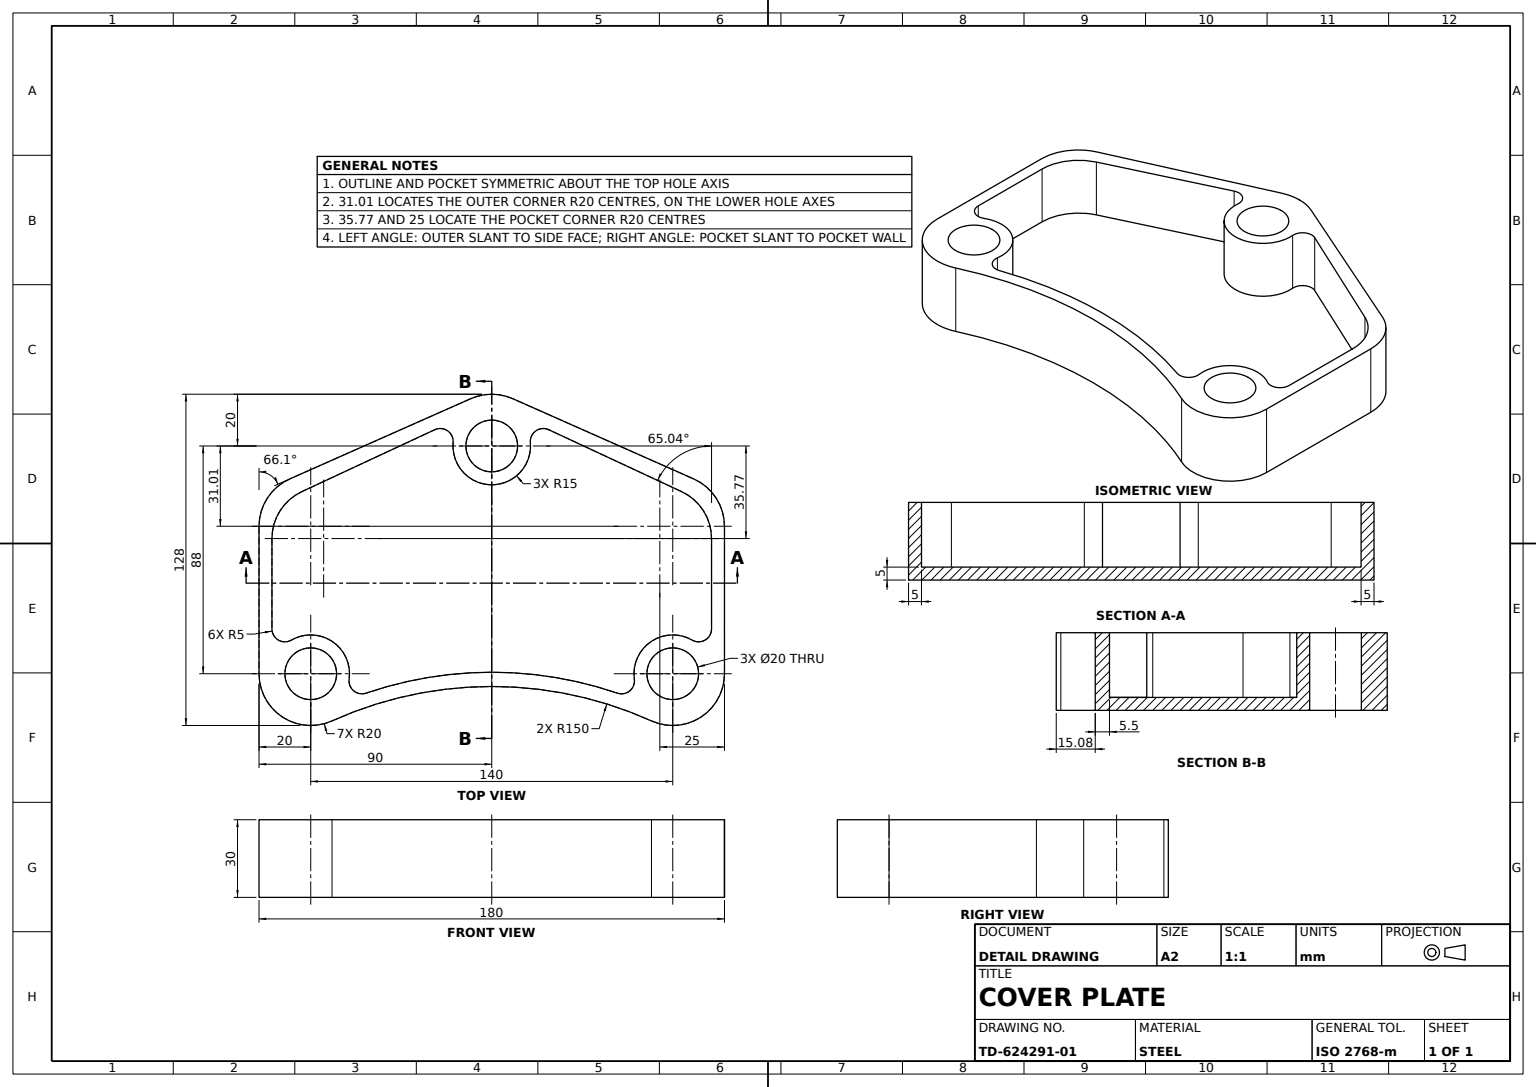
from build123d import *

# Parameters (mm, degrees)
PLATE_OUTLINE_SKETCH_R = 10
BASE_PLATE_DEPTH       = 30
POCKET_SKETCH_R        = 10
POCKET_DEPTH           = 5


with BuildPart() as part:
    # Plate Outline Sketch → Base Plate (new body)
    with BuildSketch(Plane(origin=(0, 0, 0), x_dir=(1, 0, 0), z_dir=(0, 1, 0))):
        with BuildLine():
            ThreePointArc((-90, -88), (-80.846522891, -104.803361008), (-61.764705882, -106.225803982))
            ThreePointArc((-61.764705882, -106.225803982), (0, -92.919333848), (61.764705882, -106.225803982))
            ThreePointArc((61.764705882, -106.225803982), (80.846522891, -104.803361008), (90, -88))
            Line((90, -88), (90, -31.013960492))
            ThreePointArc((90, -31.013960492), (86.763523469, -20.105968885), (78.101571911, -12.728323162))
            Line((78.101571911, -12.728323162), (8.101571911, 18.28563733))
            ThreePointArc((8.101571911, 18.28563733), (0, 20), (-8.101571911, 18.28563733))
            Line((-8.101571911, 18.28563733), (-78.101571911, -12.728323162))
            ThreePointArc((-78.101571911, -12.728323162), (-86.763523469, -20.105968885), (-90, -31.013960492))
            Line((-90, -31.013960492), (-90, -88))
        make_face()
        with Locations(Location((70, -88, 0), (0, 0, 270))):
            Circle(PLATE_OUTLINE_SKETCH_R, mode=Mode.SUBTRACT)
        with Locations(Location((-70, -88, 0), (0, 0, 270))):
            Circle(PLATE_OUTLINE_SKETCH_R, mode=Mode.SUBTRACT)
        with Locations(Location((0, 0, 0), (0, 0, 270))):
            Circle(PLATE_OUTLINE_SKETCH_R, mode=Mode.SUBTRACT)
        with BuildLine():
            ThreePointArc((55.144271878, -90.075413685), (61.617206501, -75.560997904), (77.5, -75.009618943))
            ThreePointArc((77.5, -75.009618943), (82.5, -75.009618943), (85, -70.679491924))
            Line((85, -70.679491924), (85, -35.770992672))
            ThreePointArc((85, -35.770992672), (81.864151045, -25.019229582), (73.439959048, -17.639056998))
            Line((73.439959048, -17.639056998), (22.032686199, 6.289732813))
            ThreePointArc((22.032686199, 6.289732813), (17.05201209, 5.850545589), (14.942022328, 1.317561671))
            ThreePointArc((14.942022328, 1.317561671), (0, -15), (-14.942022328, 1.317561671))
            ThreePointArc((-14.942022328, 1.317561671), (-17.05201209, 5.850545589), (-22.032686199, 6.289732813))
            Line((-22.032686199, 6.289732813), (-73.439959048, -17.639056998))
            ThreePointArc((-73.439959048, -17.639056998), (-81.864151045, -25.019229582), (-85, -35.770992672))
            Line((-85, -35.770992672), (-85, -70.679491924))
            ThreePointArc((-85, -70.679491924), (-82.5, -75.009618943), (-77.5, -75.009618943))
            ThreePointArc((-77.5, -75.009618943), (-61.617206501, -75.560997904), (-55.144271878, -90.075413685))
            ThreePointArc((-55.144271878, -90.075413685), (-53.374733144, -94.623708504), (-48.573254036, -95.497808883))
            ThreePointArc((-48.573254036, -95.497808883), (0, -87.415527975), (48.573254036, -95.497808883))
            ThreePointArc((48.573254036, -95.497808883), (53.374733144, -94.623708504), (55.144271878, -90.075413685))
        make_face(mode=Mode.SUBTRACT)
    extrude(amount=BASE_PLATE_DEPTH)

    # Pocket Sketch → Pocket (add)
    with BuildSketch(Plane.XZ):
        with BuildLine():
            Line((-90, 88), (-90, 31.013960492))
            ThreePointArc((-90, 31.013960492), (-86.763523469, 20.105968885), (-78.101571911, 12.728323162))
            Line((-78.101571911, 12.728323162), (-8.101571911, -18.28563733))
            ThreePointArc((-8.101571911, -18.28563733), (0, -20), (8.101571911, -18.28563733))
            Line((8.101571911, -18.28563733), (78.101571911, 12.728323162))
            ThreePointArc((78.101571911, 12.728323162), (86.763523469, 20.105968885), (90, 31.013960492))
            Line((90, 31.013960492), (90, 88))
            ThreePointArc((90, 88), (80.846522891, 104.803361008), (61.764705882, 106.225803982))
            ThreePointArc((61.764705882, 106.225803982), (0, 92.919333848), (-61.764705882, 106.225803982))
            ThreePointArc((-61.764705882, 106.225803982), (-80.846522891, 104.803361008), (-90, 88))
        make_face()
        with Locations(Location((-70, 88, 0), (0, 0, 90))):
            Circle(POCKET_SKETCH_R, mode=Mode.SUBTRACT)
        with Locations(Location((0, 0, 0), (0, 0, 90))):
            Circle(POCKET_SKETCH_R, mode=Mode.SUBTRACT)
        with Locations(Location((70, 88, 0), (0, 0, 90))):
            Circle(POCKET_SKETCH_R, mode=Mode.SUBTRACT)
    extrude(amount=-POCKET_DEPTH)


solid = part.part
